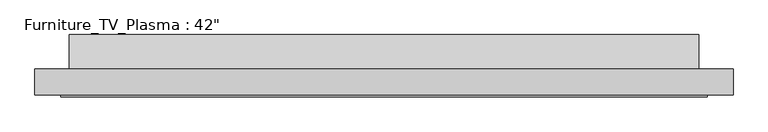
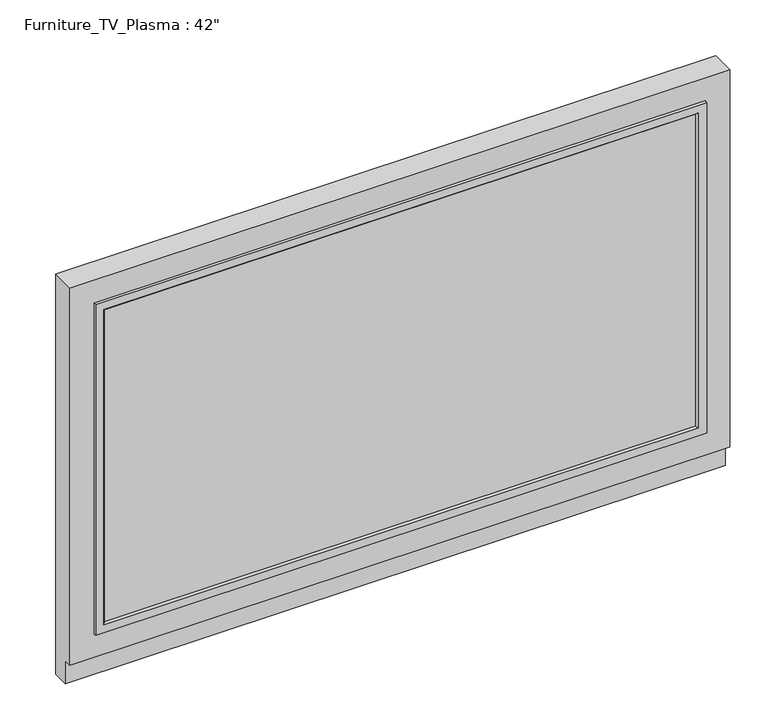
"""IFC4 building model written with IfcOpenShell, lengths in millimetres: furniture geometry."""

from ifc_helpers import new_model, si_unit, frame, origin, place, context, project, spatial, polyline, outline, extrude, faceted_brep, source, transform, mapped, element, save


def furniture_0b97a49d(model_context):
    return source(origin(), model_context, "Body", "SolidModel", [
        faceted_brep([(571.5, -50.8, 660.4), (-457.2, -50.8, 660.4), (-457.2, -88.9, 660.4), (571.5, -88.9, 660.4), (-457.2, -50.8, 0.0), (571.5, -50.8, 0.0), (571.5, -76.2, 0.0), (-457.2, -76.2, 0.0), (-457.2, -76.2, 38.1), (-457.2, -88.9, 38.1), (571.5, -88.9, 38.1), (533.4, -88.9, 622.3), (533.4, -88.9, 76.2), (-419.1, -88.9, 76.2), (-419.1, -88.9, 622.3), (571.5, -76.2, 38.1), (533.4, -74.1720413, 622.3), (-419.1, -74.1720413, 622.3), (-419.1, -74.1720413, 76.2), (533.4, -74.1720413, 76.2)], [[[0, 1, 2, 3]], [[4, 5, 6, 7]], [[1, 0, 5, 4]], [[2, 1, 4, 7, 8, 9]], [[3, 2, 9, 10], [11, 12, 13, 14]], [[0, 3, 10, 15, 6, 5]], [[16, 17, 18, 19]], [[16, 19, 12, 11]], [[19, 18, 13, 12]], [[18, 17, 14, 13]], [[17, 16, 11, 14]], [[15, 8, 7, 6]], [[8, 15, 10, 9]]]),
        extrude(outline(polyline([(520.7, -88.9), (-406.4, -88.9), (-406.4, -74.1720413), (520.7, -74.1720413), (520.7, -88.9)])), frame((0.0, 0.0, 88.9), z_axis=(0.0, 0.0, 1.0), x_axis=(1.0, 0.0, 0.0)), (0.0, 0.0, 1.0), 520.7),
        extrude(outline(polyline([(0.0, 574.8688953), (0.0, 38.1), (-50.8, 38.1), (-50.8, 609.6), (0.0, 574.8688953)])), frame((-406.4, 0.0, 0.0), z_axis=(1.0, 0.0, 0.0), x_axis=(0.0, 1.0, 0.0)), (0.0, 0.0, 1.0), 927.1),
        faceted_brep([(517.525, -88.9, 92.075), (520.7, -92.075, 88.9), (520.7, -92.075, 608.80625), (517.525, -88.9, 605.63125), (520.7, -74.1720413, 88.9), (520.7, -88.9, 88.9), (520.7, -88.9, 608.80625), (520.7, -74.1720413, 608.80625), (533.4, -92.075, 76.2), (533.4, -74.1720413, 76.2), (533.4, -74.1720413, 621.50625), (533.4, -92.075, 621.50625), (-406.4, -92.075, 608.80625), (-403.225, -88.9, 605.63125), (-406.4, -88.9, 608.80625), (-406.4, -74.1720413, 608.80625), (-419.1, -74.1720413, 621.50625), (-419.1, -92.075, 621.50625), (-406.4, -92.075, 88.9), (-403.225, -88.9, 92.075), (-406.4, -88.9, 88.9), (-406.4, -74.1720413, 88.9), (-419.1, -74.1720413, 76.2), (-419.1, -92.075, 76.2)], [[[0, 1, 2, 3]], [[4, 5, 6, 7]], [[8, 9, 10, 11]], [[3, 2, 12, 13]], [[7, 6, 14, 15]], [[11, 10, 16, 17]], [[13, 12, 18, 19]], [[15, 14, 20, 21]], [[17, 16, 22, 23]], [[11, 17, 23, 8], [1, 18, 12, 2]], [[19, 18, 1, 0]], [[5, 20, 14, 6], [3, 13, 19, 0]], [[21, 20, 5, 4]], [[9, 22, 16, 10], [7, 15, 21, 4]], [[23, 22, 9, 8]]]),
    ])


if __name__ == "__main__":
    model = new_model("IFC4")
    model_context = context("Model", 3, world=origin())
    ifc_project = project(units=[si_unit("LENGTHUNIT", "METRE", prefix="MILLI")], contexts=[model_context])
    site = spatial("IfcSite", under=ifc_project)
    building = spatial("IfcBuilding", under=site)
    placement = place(None, origin())
    furniture_shape = furniture_0b97a49d(model_context)
    element("IfcFurniture", 1, ObjectType="Furniture_TV_Plasma : 42\"", at=placement, inside=building, context=model_context, shape_type="MappedRepresentation", body=[
        mapped(furniture_shape, transform((0.0, 0.0, 0.0), x_axis=(1.0, 0.0, 0.0), y_axis=(0.0, 1.0, 0.0), z_axis=(0.0, 0.0, 1.0))),
    ])
    save(model, "model.ifc")

# Revit data of these elements
# Type "Furniture_TV_Plasma : 42\""
#   Keynote = "N"
#   Assembly Code = "E2020200"
#   Depth = 88.9 mm
#   Height = 660.4 mm
#   Width = 1028.7 mm
#   Material Cabinet = Plastic - Gray
#   Default Elevation = 0
# Element 1 (IfcFurniture, "Furniture_TV_Plasma : 42\"")
#   Materials on its faces: "Plastic - Black", "Plastic - Gray", "Glass"
# Materials
#   "Plastic - Gray": class "Plastic", colour RGB 134 134 134, transparency 0
#   "Plastic - Black": colour RGB 0 0 0, transparency 0
#   "Glass": class "Glass", colour RGB 0 128 192, transparency 0.9, Description = "Soda Lime Glass", Cost = 0
